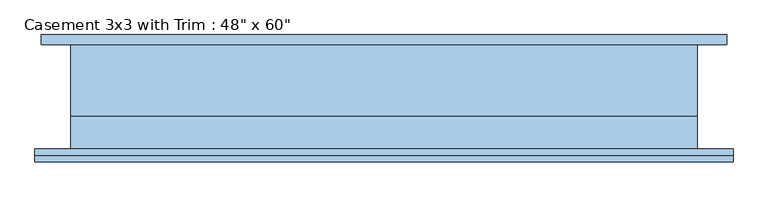
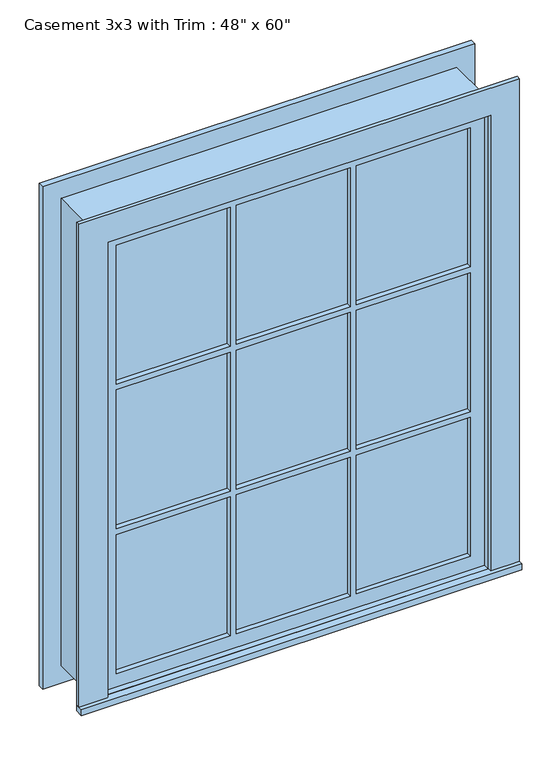
"""IFC4 building model written with IfcOpenShell, lengths in millimetres: window geometry."""

from ifc_helpers import new_model, si_unit, frame, origin, place, context, project, spatial, polyline, outline, extrude, source, transform, mapped, element, save


def window_2b070d82(model_context):
    return source(origin(), model_context, "Body", "SweptSolid", [
        extrude(outline(polyline([(-679.45, -127.0), (-679.45, -101.6), (679.45, -101.6), (679.45, -127.0), (-679.45, -127.0)])), frame((0.0, 0.0, 304.8), z_axis=(0.0, 0.0, 1.0), x_axis=(1.0, 0.0, 0.0)), (0.0, 0.0, 1.0), 19.05),
        extrude(outline(polyline([(1809.75, -590.55), (1809.75, 590.55), (323.85, 590.55), (323.85, 679.45), (1898.65, 679.45), (1898.65, -679.45), (323.85, -679.45), (323.85, -590.55), (1809.75, -590.55)])), frame((0.0, -114.3, 0.0), z_axis=(0.0, 1.0, 0.0), x_axis=(0.0, 0.0, 1.0)), (0.0, 0.0, 1.0), 12.7),
        extrude(outline(polyline([(194.7333333, -66.675), (194.7333333, -53.975), (546.1, -53.975), (546.1, -66.675), (194.7333333, -66.675)])), frame((0.0, 0.0, 1312.3333333), z_axis=(0.0, 0.0, 1.0), x_axis=(1.0, 0.0, 0.0)), (0.0, 0.0, 1.0), 452.9666667),
        extrude(outline(polyline([(-175.6833333, -66.675), (-175.6833333, -53.975), (175.6833333, -53.975), (175.6833333, -66.675), (-175.6833333, -66.675)])), frame((0.0, 0.0, 1312.3333333), z_axis=(0.0, 0.0, 1.0), x_axis=(1.0, 0.0, 0.0)), (0.0, 0.0, 1.0), 452.9666667),
        extrude(outline(polyline([(-546.1, -66.675), (-546.1, -53.975), (-194.7333333, -53.975), (-194.7333333, -66.675), (-546.1, -66.675)])), frame((0.0, 0.0, 1312.3333333), z_axis=(0.0, 0.0, 1.0), x_axis=(1.0, 0.0, 0.0)), (0.0, 0.0, 1.0), 452.9666667),
        extrude(outline(polyline([(-546.1, -66.675), (-546.1, -53.975), (-194.7333333, -53.975), (-194.7333333, -66.675), (-546.1, -66.675)])), frame((0.0, 0.0, 840.3166667), z_axis=(0.0, 0.0, 1.0), x_axis=(1.0, 0.0, 0.0)), (0.0, 0.0, 1.0), 452.9666667),
        extrude(outline(polyline([(-175.6833333, -66.675), (-175.6833333, -53.975), (175.6833333, -53.975), (175.6833333, -66.675), (-175.6833333, -66.675)])), frame((0.0, 0.0, 840.3166667), z_axis=(0.0, 0.0, 1.0), x_axis=(1.0, 0.0, 0.0)), (0.0, 0.0, 1.0), 452.9666667),
        extrude(outline(polyline([(194.7333333, -66.675), (194.7333333, -53.975), (546.1, -53.975), (546.1, -66.675), (194.7333333, -66.675)])), frame((0.0, 0.0, 840.3166667), z_axis=(0.0, 0.0, 1.0), x_axis=(1.0, 0.0, 0.0)), (0.0, 0.0, 1.0), 452.9666667),
        extrude(outline(polyline([(194.7333333, -66.675), (194.7333333, -53.975), (546.1, -53.975), (546.1, -66.675), (194.7333333, -66.675)])), frame((0.0, 0.0, 368.3), z_axis=(0.0, 0.0, 1.0), x_axis=(1.0, 0.0, 0.0)), (0.0, 0.0, 1.0), 452.9666667),
        extrude(outline(polyline([(-175.6833333, -66.675), (-175.6833333, -53.975), (175.6833333, -53.975), (175.6833333, -66.675), (-175.6833333, -66.675)])), frame((0.0, 0.0, 368.3), z_axis=(0.0, 0.0, 1.0), x_axis=(1.0, 0.0, 0.0)), (0.0, 0.0, 1.0), 452.9666667),
        extrude(outline(polyline([(-546.1, -66.675), (-546.1, -53.975), (-194.7333333, -53.975), (-194.7333333, -66.675), (-546.1, -66.675)])), frame((0.0, 0.0, 368.3), z_axis=(0.0, 0.0, 1.0), x_axis=(1.0, 0.0, 0.0)), (0.0, 0.0, 1.0), 452.9666667),
        extrude(outline(polyline([(1885.95, 666.75), (1885.95, -666.75), (247.65, -666.75), (247.65, 666.75), (1885.95, 666.75)]), holes=[polyline([(1797.05, 577.85), (336.55, 577.85), (336.55, -577.85), (1797.05, -577.85), (1797.05, 577.85)])]), frame((0.0, 101.6, 0.0), z_axis=(0.0, 1.0, 0.0), x_axis=(0.0, 0.0, 1.0)), (0.0, 0.0, 1.0), 19.05),
        extrude(outline(polyline([(1809.75, -590.55), (323.85, -590.55), (323.85, 590.55), (1809.75, 590.55), (1809.75, -590.55)]), holes=[polyline([(1765.3, -194.7333333), (1312.3333333, -194.7333333), (1312.3333333, -546.1), (1765.3, -546.1), (1765.3, -194.7333333)]), polyline([(1293.2833333, -194.7333333), (840.3166667, -194.7333333), (840.3166667, -546.1), (1293.2833333, -546.1), (1293.2833333, -194.7333333)]), polyline([(821.2666667, -194.7333333), (368.3, -194.7333333), (368.3, -546.1), (821.2666667, -546.1), (821.2666667, -194.7333333)]), polyline([(1765.3, 175.6833333), (1312.3333333, 175.6833333), (1312.3333333, -175.6833333), (1765.3, -175.6833333), (1765.3, 175.6833333)]), polyline([(1293.2833333, 175.6833333), (840.3166667, 175.6833333), (840.3166667, -175.6833333), (1293.2833333, -175.6833333), (1293.2833333, 175.6833333)]), polyline([(821.2666667, 175.6833333), (368.3, 175.6833333), (368.3, -175.6833333), (821.2666667, -175.6833333), (821.2666667, 175.6833333)]), polyline([(1765.3, 546.1), (1312.3333333, 546.1), (1312.3333333, 194.7333333), (1765.3, 194.7333333), (1765.3, 546.1)]), polyline([(1293.2833333, 546.1), (840.3166667, 546.1), (840.3166667, 194.7333333), (1293.2833333, 194.7333333), (1293.2833333, 546.1)]), polyline([(821.2666667, 546.1), (368.3, 546.1), (368.3, 194.7333333), (821.2666667, 194.7333333), (821.2666667, 546.1)])]), frame((0.0, -82.55, 0.0), z_axis=(0.0, 1.0, 0.0), x_axis=(0.0, 0.0, 1.0)), (0.0, 0.0, 1.0), 44.45),
        extrude(outline(polyline([(1828.8, -609.6), (304.8, -609.6), (304.8, 609.6), (1828.8, 609.6), (1828.8, -609.6)]), holes=[polyline([(1797.05, -577.85), (1797.05, 577.85), (336.55, 577.85), (336.55, -577.85), (1797.05, -577.85)])]), frame((0.0, -38.1, 0.0), z_axis=(0.0, 1.0, 0.0), x_axis=(0.0, 0.0, 1.0)), (0.0, 0.0, 1.0), 139.7),
        extrude(outline(polyline([(1828.8, 609.6), (1828.8, -609.6), (304.8, -609.6), (304.8, 609.6), (1828.8, 609.6)]), holes=[polyline([(1809.75, 590.55), (323.85, 590.55), (323.85, -590.55), (1809.75, -590.55), (1809.75, 590.55)])]), frame((0.0, -101.6, 0.0), z_axis=(0.0, 1.0, 0.0), x_axis=(0.0, 0.0, 1.0)), (0.0, 0.0, 1.0), 63.5),
    ])


if __name__ == "__main__":
    model = new_model("IFC4")
    model_context = context("Model", 3, world=origin())
    ifc_project = project(units=[si_unit("LENGTHUNIT", "METRE", prefix="MILLI")], contexts=[model_context])
    site = spatial("IfcSite", under=ifc_project)
    building = spatial("IfcBuilding", under=site)
    placement = place(None, origin())
    window_shape = window_2b070d82(model_context)
    element("IfcWindow", 1, ObjectType="Casement 3x3 with Trim : 48\" x 60\"", at=placement, inside=building, context=model_context, shape_type="MappedRepresentation", body=[
        mapped(window_shape, transform((0.0, 0.0, 0.0), x_axis=(1.0, 0.0, 0.0), y_axis=(0.0, 1.0, 0.0), z_axis=(0.0, 0.0, 1.0))),
    ])
    save(model, "model.ifc")

# Revit data of these elements
# Type "Casement 3x3 with Trim : 48\" x 60\""
#   Type Mark = "12"
#   Construction Type Id = "GSP4R"
#   Assembly Code = "B2020100"
#   Analytic Construction = "1/8 in Pilkington single glazing"
#   Visual Light Transmittance = 0.9
#   Solar Heat Gain Coefficient = 0.78
#   Heat Transfer Coefficient (U) = 0.6496 BTU/(h·ft²·°F)
#   Height = 5' - 0"
#   Default Sill Height = 1' - 0"
#   Trim Projection - Ext. = 0' - 0 1/2"
#   Trim Projection - Int. = 0' - 0 3/4"
#   Trim Width - Exterior = 0' - 3 1/2"
#   Trim Width - Interior = 0' - 3 1/2"
#   Width = 4' - 0"
#   Window Inset = 0' - 0 3/4"
#   Define Thermal Properties by = 1
#   Glass Pane Material = Glass
#   Sash Material = Sash
#   Trim Exterior Material = Trim
#   Trim Interior Material = Trim
#   Wall Closure = (empty or 0)
# Element 1 (IfcWindow, "Casement 3x3 with Trim : 48\" x 60\"")
#   Materials on its faces: "Sash", "Glass", "Trim"
# Materials
#   "Glass": class "Glass", colour RGB 0 128 192, transparency 0.75, Description = "Soda Lime Glass", Cost = 0
#   "Sash": class "Wood", colour RGB 224 178 126, transparency 0
#   "Trim": class "Wood", colour RGB 224 178 126, transparency 0
